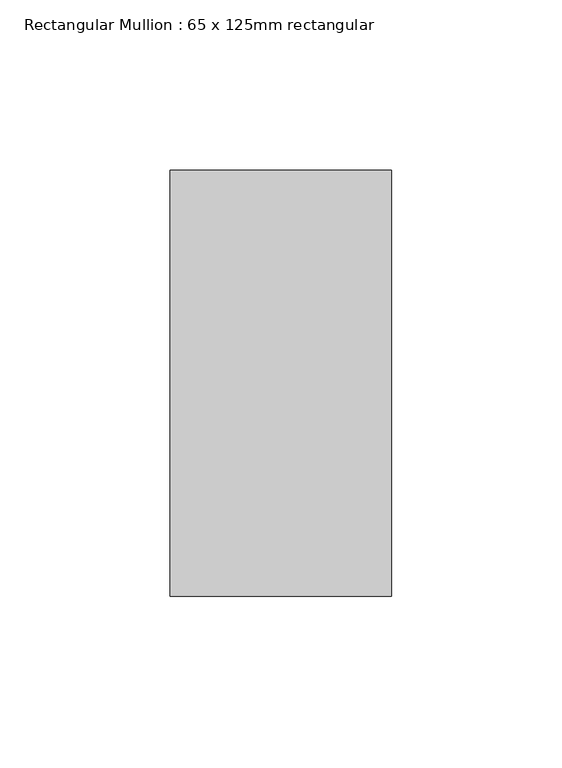
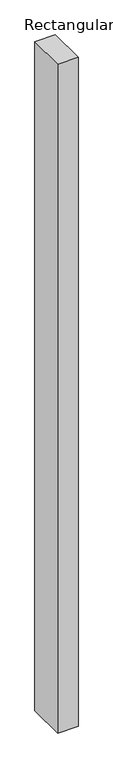
"""IFC4 building model written with IfcOpenShell, lengths in millimetres: member geometry, Rectangular Mullion : 65 x 125mm rectangular."""

from ifc_helpers import new_model, si_unit, frame, origin, place, context, project, spatial, polyline, outline, extrude, source, transform, mapped, element, save


def rectangular_mullion_65_x_125mm_rectangular_c9dcdcb6(model_context):
    return source(origin(), model_context, "Body", "SweptSolid", [
        extrude(outline(polyline([(0.0, 62.5), (0.0, -62.5), (-65.0, -62.5), (-65.0, 62.5), (0.0, 62.5)])), frame((0.0, 0.0, -2250.0), z_axis=(0.0, 0.0, 1.0), x_axis=(1.0, 0.0, 0.0)), (0.0, 0.0, 1.0), 2250.0),
    ])


if __name__ == "__main__":
    model = new_model("IFC4")
    model_context = context("Model", 3, world=origin())
    ifc_project = project(units=[si_unit("LENGTHUNIT", "METRE", prefix="MILLI")], contexts=[model_context])
    site = spatial("IfcSite", under=ifc_project)
    building = spatial("IfcBuilding", under=site)
    placement = place(None, origin())
    rectangular_mullion_65_x_125mm_rectangular_shape = rectangular_mullion_65_x_125mm_rectangular_c9dcdcb6(model_context)
    element("IfcMember", 1, ObjectType="Rectangular Mullion : 65 x 125mm rectangular", at=placement, inside=building, context=model_context, shape_type="MappedRepresentation", body=[
        mapped(rectangular_mullion_65_x_125mm_rectangular_shape, transform((0.0, 0.0, 0.0), x_axis=(1.0, 0.0, 0.0), y_axis=(0.0, 1.0, 0.0), z_axis=(0.0, 0.0, 1.0))),
    ])
    save(model, "model.ifc")

# Revit data of these elements
# Type "Rectangular Mullion : 65 x 125mm rectangular"
#   built-in parameter 1007304 = 0.410105 (stored number, unit not read)
#   built-in parameter 1007301 = 0.106627 (stored number, unit not read)
#   built-in parameter 1007300 = 0.106627 (stored number, unit not read)
# Element 1 (IfcMember, "Rectangular Mullion : 65 x 125mm rectangular")
#   Materials on its faces: "Aluminum"
# Materials
#   "Aluminum": class "Metal", colour RGB 244 245 246, transparency 0, Description = "Aluminum 6061", Cost = 0
